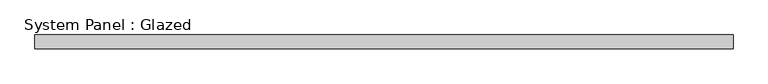
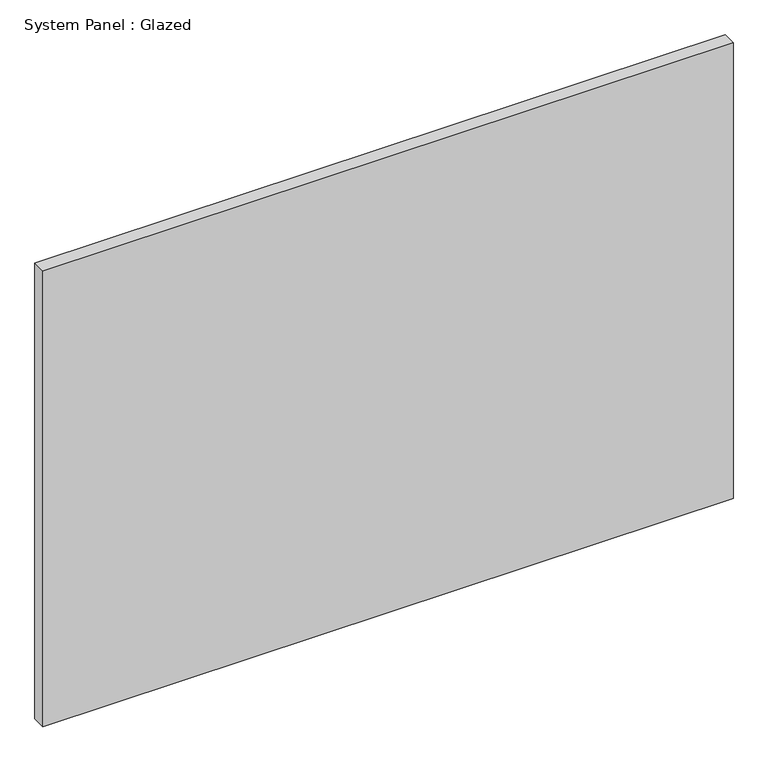
"""IFC4 building model written with IfcOpenShell, lengths in millimetres: plate geometry, System Panel : Glazed."""

from ifc_helpers import new_model, si_unit, origin, origin_with_axes, place, context, project, spatial, polyline, outline, extrude, source, transform, mapped, element, save


def system_panel_glazed_0daebeb7(model_context):
    return source(origin(), model_context, "Body", "SweptSolid", [
        extrude(outline(polyline([(638.175, 19.05), (-638.175, 19.05), (-638.175, 44.45), (638.175, 44.45), (638.175, 19.05)])), origin_with_axes(), (0.0, 0.0, 1.0), 890.928642),
    ])


if __name__ == "__main__":
    model = new_model("IFC4")
    model_context = context("Model", 3, world=origin())
    ifc_project = project(units=[si_unit("LENGTHUNIT", "METRE", prefix="MILLI")], contexts=[model_context])
    site = spatial("IfcSite", under=ifc_project)
    building = spatial("IfcBuilding", under=site)
    placement = place(None, origin())
    system_panel_glazed_shape = system_panel_glazed_0daebeb7(model_context)
    element("IfcPlate", 1, ObjectType="System Panel : Glazed", at=placement, inside=building, context=model_context, shape_type="MappedRepresentation", body=[
        mapped(system_panel_glazed_shape, transform((0.0, 0.0, 0.0), x_axis=(1.0, 0.0, 0.0), y_axis=(0.0, 1.0, 0.0), z_axis=(0.0, 0.0, 1.0))),
    ])
    save(model, "model.ifc")

# Revit data of these elements
# Type "System Panel : Glazed"
#   Construction Type Id = "GSP4R"
#   Analytic Construction = "1/8 in Pilkington single glazing"
#   Visual Light Transmittance = 0.9
#   Solar Heat Gain Coefficient = 0.86
#   Heat Transfer Coefficient (U) = 1.18115 BTU/(h·ft²·°F)
#   Define Thermal Properties by = 1
# Element 1 (IfcPlate, "System Panel : Glazed")
#   Materials on its faces: "Glass"
# Materials
#   "Glass": class "Glass", colour RGB 0 128 192, transparency 0.75, Description = "Soda Lime Glass", Cost = 0
